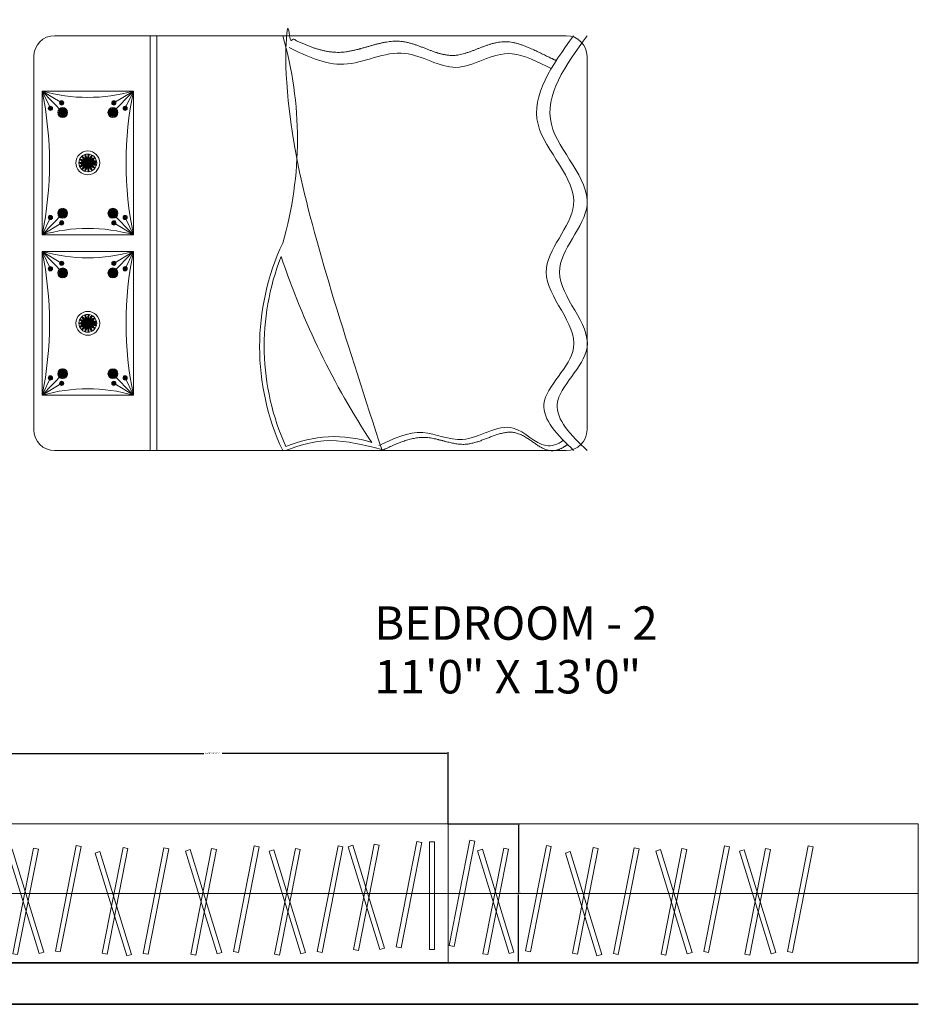
# Model space of a CAD drawing. Units: inches. Extents: x -61 to 1599, y -1316 to 257.
# Tile 74 of 204: x 406 to 536, y -788 to -646. Entities that reach past the tile are written whole.
import ezdxf

# ---------------------------------------------------------------- set-up
doc = ezdxf.new("R2010")
doc.units = ezdxf.units.IN
doc.header["$MEASUREMENT"] = 0
for name, color, linetype, lineweight in [('A-ANNO-DIMS', 2, 'Continuous', 18), ('A-AREA-IDEN', 1, 'Continuous', 18), ('A-FLOR-CASE', 8, 'Continuous', 18), ('FURNITURE', 83, 'Continuous', 18), ('WALLS', 4, 'Continuous', 35)]:
    doc.layers.add(name, color=color, linetype=linetype, lineweight=lineweight)
doc.layers.add('LT', color=8, linetype='Continuous')
doc.styles.get("Standard").update_dxf_attribs({"font": 'arial.ttf'})
doc.dimstyles.get("Standard").update_dxf_attribs({"dimtxt": 0.18, "dimasz": 0.18, "dimexe": 0.18, "dimexo": 0.0625, "dimgap": 0.09, "dimtad": 0, "dimtih": 1, "dimtoh": 1, "dimdec": 0, "dimzin": 0, "dimdsep": 46, "dimlunit": 3, "dimtxsty": 'Standard', "dimcen": 0.09, "dimadec": 0, "dimazin": 0, "dimtfac": 1, "dimtdec": 0, "dimtofl": 0, "dimtmove": 0, "dimatfit": 3, "dimfxl": 1, "dimtolj": 1, "dimtzin": 0, "dimarcsym": 0})

# ---------------------------------------------------------------- blocks, each defined once
blk = doc.blocks.new('*U324')
at = {"layer": 'LT'}
blk.add_line((0, 0.64), (0, -0.64), dxfattribs=at)
for centre, start, end in [((1.87, 0), 160.9983, 199.0017), ((-1.87, 0), 340.9983, 19.0017)]:
    blk.add_arc(centre, 1.97, start, end, dxfattribs=at)
blk = doc.blocks.new('*U311')
at = {"layer": 'FURNITURE', "transparency": 16777216}
for p, rotation in [((-244.2, -68.53), 48.00000000000001), ((-243.98, -68.38), 23.99999999999999), ((-243.46, -68.38), 336.0000000000001), ((-243.25, -68.53), 312), ((-244.36, -69.03), 96), ((-244.33, -68.76), 72), ((-244.28, -69.28), 120), ((-244.1, -69.48), 144), ((-243.86, -69.59), 168), ((-243.59, -69.59), 192), ((-243.34, -69.48), 216), ((-243.17, -69.28), 240), ((-243.11, -68.76), 288), ((-243.08, -69.03), 264)]:
    blk.add_blockref('*U324', p, dxfattribs=dict(at, rotation=rotation))
blk.add_blockref('*U324', (-243.72, -68.32), dxfattribs=at)
blk = doc.blocks.new('*U312')
at = {"layer": 'LT'}
blk.add_line((0, 0.36), (0, -0.36), dxfattribs=at)
for centre, start, end in [((1.04, 0), 160.9983, 199.0017), ((-1.04, 0), 340.9983, 19.0017)]:
    blk.add_arc(centre, 1.1, start, end, dxfattribs=at)
blk = doc.blocks.new('*U313')
at = {"layer": 'FURNITURE', "transparency": 16777216}
for p, rotation in [((-136.32, -38.51), 96), ((-136.3, -38.36), 72), ((-136.27, -38.65), 120), ((-136.23, -38.23), 48.00000000000001), ((-136.17, -38.76), 144), ((-136.11, -38.14), 23.99999999999999), ((-135.82, -38.14), 336.0000000000001), ((-135.75, -38.76), 216), ((-135.69, -38.23), 312), ((-135.65, -38.65), 240), ((-135.62, -38.36), 288.0000000000001), ((-135.6, -38.51), 264), ((-136.04, -38.82), 168.0000000000001), ((-135.89, -38.82), 191.9999999999999)]:
    blk.add_blockref('*U312', p, dxfattribs=dict(at, rotation=rotation))
blk.add_blockref('*U312', (-135.96, -38.11), dxfattribs=at)
blk = doc.blocks.new('*U318')
at = {"layer": 'LT'}
blk.add_line((0, 0.15), (0, -0.15), dxfattribs=at)
for centre, start, end in [((0.44, 0), 160.9983, 199.0017), ((-0.44, 0), 340.9983, 19.0017)]:
    blk.add_arc(centre, 0.468, start, end, dxfattribs=at)
blk = doc.blocks.new('*U319')
at = {"layer": 'FURNITURE', "transparency": 16777216}
for p, rotation in [((-57.96, -16.37), 96), ((-57.96, -16.31), 72), ((-57.94, -16.43), 120), ((-57.93, -16.26), 48.00000000000001), ((-57.9, -16.48), 144), ((-57.87, -16.22), 24), ((-57.84, -16.51), 168.0000000000001), ((-57.75, -16.22), 336), ((-57.78, -16.51), 192), ((-57.7, -16.26), 312), ((-57.72, -16.48), 216), ((-57.68, -16.43), 240), ((-57.67, -16.31), 288), ((-57.66, -16.37), 264)]:
    blk.add_blockref('*U318', p, dxfattribs=dict(at, rotation=rotation))
blk.add_blockref('*U318', (-57.81, -16.21), dxfattribs=at)
blk = doc.blocks.new('*U320')
at = {"layer": 'LT'}
blk.add_line((0, 0.15), (0, -0.15), dxfattribs=at)
for centre, start, end in [((0.44, 0), 160.9983, 199.0017), ((-0.44, 0), 340.9983, 19.0017)]:
    blk.add_arc(centre, 0.468, start, end, dxfattribs=at)
blk = doc.blocks.new('*U321')
at = {"layer": 'FURNITURE', "transparency": 16777216}
for p, rotation in [((-57.96, -16.37), 96), ((-57.96, -16.31), 72), ((-57.94, -16.43), 120), ((-57.93, -16.26), 48.00000000000001), ((-57.9, -16.48), 144), ((-57.87, -16.22), 24), ((-57.84, -16.51), 168.0000000000001), ((-57.75, -16.22), 336), ((-57.78, -16.51), 192), ((-57.7, -16.26), 312), ((-57.72, -16.48), 216), ((-57.68, -16.43), 240), ((-57.67, -16.31), 288), ((-57.66, -16.37), 264)]:
    blk.add_blockref('*U320', p, dxfattribs=dict(at, rotation=rotation))
blk.add_blockref('*U320', (-57.81, -16.21), dxfattribs=at)
blk = doc.blocks.new('*U275')
at = {"layer": 'LT'}
blk.add_line((0, 0.36), (0, -0.36), dxfattribs=at)
for centre, start, end in [((1.04, 0), 160.9983, 199.0017), ((-1.04, 0), 340.9983, 19.0017)]:
    blk.add_arc(centre, 1.1, start, end, dxfattribs=at)
blk = doc.blocks.new('*U317')
at = {"layer": 'FURNITURE', "transparency": 16777216}
for p, rotation in [((-136.32, -38.51), 96), ((-136.3, -38.36), 72), ((-136.27, -38.65), 120), ((-136.23, -38.23), 48.00000000000001), ((-136.17, -38.76), 144), ((-136.11, -38.14), 23.99999999999999), ((-135.82, -38.14), 336.0000000000001), ((-135.75, -38.76), 216), ((-135.69, -38.23), 312), ((-135.65, -38.65), 240), ((-135.62, -38.36), 288.0000000000001), ((-135.6, -38.51), 264), ((-136.04, -38.82), 168.0000000000001), ((-135.89, -38.82), 191.9999999999999)]:
    blk.add_blockref('*U275', p, dxfattribs=dict(at, rotation=rotation))
blk.add_blockref('*U275', (-135.96, -38.11), dxfattribs=at)
blk = doc.blocks.new('*U322')
at = {"layer": 'LT'}
blk.add_line((0, 0.15), (0, -0.15), dxfattribs=at)
for centre, start, end in [((0.44, 0), 160.9983, 199.0017), ((-0.44, 0), 340.9983, 19.0017)]:
    blk.add_arc(centre, 0.468, start, end, dxfattribs=at)
blk = doc.blocks.new('*U323')
at = {"layer": 'FURNITURE', "transparency": 16777216}
for p, rotation in [((-57.96, -16.37), 96), ((-57.96, -16.31), 72), ((-57.94, -16.43), 120), ((-57.93, -16.26), 48.00000000000001), ((-57.9, -16.48), 144), ((-57.87, -16.22), 24), ((-57.84, -16.51), 168.0000000000001), ((-57.75, -16.22), 336), ((-57.78, -16.51), 192), ((-57.7, -16.26), 312), ((-57.72, -16.48), 216), ((-57.68, -16.43), 240), ((-57.67, -16.31), 288), ((-57.66, -16.37), 264)]:
    blk.add_blockref('*U322', p, dxfattribs=dict(at, rotation=rotation))
blk.add_blockref('*U322', (-57.81, -16.21), dxfattribs=at)
blk = doc.blocks.new('*U273')
at = {"layer": 'LT'}
blk.add_line((0, 0.15), (0, -0.15), dxfattribs=at)
for centre, start, end in [((0.44, 0), 160.9983, 199.0017), ((-0.44, 0), 340.9983, 19.0017)]:
    blk.add_arc(centre, 0.468, start, end, dxfattribs=at)
blk = doc.blocks.new('*U274')
at = {"layer": 'FURNITURE', "transparency": 16777216}
for p, rotation in [((-57.96, -16.37), 96), ((-57.96, -16.31), 72), ((-57.94, -16.43), 120), ((-57.93, -16.26), 48.00000000000001), ((-57.9, -16.48), 144), ((-57.87, -16.22), 24), ((-57.84, -16.51), 168.0000000000001), ((-57.75, -16.22), 336), ((-57.78, -16.51), 192), ((-57.7, -16.26), 312), ((-57.72, -16.48), 216), ((-57.68, -16.43), 240), ((-57.67, -16.31), 288), ((-57.66, -16.37), 264)]:
    blk.add_blockref('*U273', p, dxfattribs=dict(at, rotation=rotation))
blk.add_blockref('*U273', (-57.81, -16.21), dxfattribs=at)
blk = doc.blocks.new('*U301')
at = {"layer": 'LT'}
blk.add_line((0, 0.36), (0, -0.36), dxfattribs=at)
for centre, start, end in [((1.04, 0), 160.9983, 199.0017), ((-1.04, 0), 340.9983, 19.0017)]:
    blk.add_arc(centre, 1.1, start, end, dxfattribs=at)
blk = doc.blocks.new('*U302')
at = {"layer": 'FURNITURE', "transparency": 16777216}
for p, rotation in [((-136.32, -38.51), 96), ((-136.3, -38.36), 72), ((-136.27, -38.65), 120), ((-136.23, -38.23), 48.00000000000001), ((-136.17, -38.76), 144), ((-136.11, -38.14), 23.99999999999999), ((-135.82, -38.14), 336.0000000000001), ((-135.75, -38.76), 216), ((-135.69, -38.23), 312), ((-135.65, -38.65), 240), ((-135.62, -38.36), 288.0000000000001), ((-135.6, -38.51), 264), ((-136.04, -38.82), 168.0000000000001), ((-135.89, -38.82), 191.9999999999999)]:
    blk.add_blockref('*U301', p, dxfattribs=dict(at, rotation=rotation))
blk.add_blockref('*U301', (-135.96, -38.11), dxfattribs=at)
blk = doc.blocks.new('*U294')
at = {"layer": 'LT'}
blk.add_line((0, 0.15), (0, -0.15), dxfattribs=at)
for centre, start, end in [((0.44, 0), 160.9983, 199.0017), ((-0.44, 0), 340.9983, 19.0017)]:
    blk.add_arc(centre, 0.468, start, end, dxfattribs=at)
blk = doc.blocks.new('*U295')
at = {"layer": 'FURNITURE', "transparency": 16777216}
for p, rotation in [((-57.96, -16.37), 96), ((-57.96, -16.31), 72), ((-57.94, -16.43), 120), ((-57.93, -16.26), 48.00000000000001), ((-57.9, -16.48), 144), ((-57.87, -16.22), 24), ((-57.84, -16.51), 168.0000000000001), ((-57.75, -16.22), 336), ((-57.78, -16.51), 192), ((-57.7, -16.26), 312), ((-57.72, -16.48), 216), ((-57.68, -16.43), 240), ((-57.67, -16.31), 288), ((-57.66, -16.37), 264)]:
    blk.add_blockref('*U294', p, dxfattribs=dict(at, rotation=rotation))
blk.add_blockref('*U294', (-57.81, -16.21), dxfattribs=at)
blk = doc.blocks.new('*U296')
at = {"layer": 'LT'}
blk.add_line((0, 0.15), (0, -0.15), dxfattribs=at)
for centre, start, end in [((0.44, 0), 160.9983, 199.0017), ((-0.44, 0), 340.9983, 19.0017)]:
    blk.add_arc(centre, 0.468, start, end, dxfattribs=at)
blk = doc.blocks.new('*U297')
at = {"layer": 'FURNITURE', "transparency": 16777216}
for p, rotation in [((-57.96, -16.37), 96), ((-57.96, -16.31), 72), ((-57.94, -16.43), 120), ((-57.93, -16.26), 48.00000000000001), ((-57.9, -16.48), 144), ((-57.87, -16.22), 24), ((-57.84, -16.51), 168.0000000000001), ((-57.75, -16.22), 336), ((-57.78, -16.51), 192), ((-57.7, -16.26), 312), ((-57.72, -16.48), 216), ((-57.68, -16.43), 240), ((-57.67, -16.31), 288), ((-57.66, -16.37), 264)]:
    blk.add_blockref('*U296', p, dxfattribs=dict(at, rotation=rotation))
blk.add_blockref('*U296', (-57.81, -16.21), dxfattribs=at)
blk = doc.blocks.new('*U292')
at = {"layer": 'LT'}
blk.add_line((0, 0.36), (0, -0.36), dxfattribs=at)
for centre, start, end in [((1.04, 0), 160.9983, 199.0017), ((-1.04, 0), 340.9983, 19.0017)]:
    blk.add_arc(centre, 1.1, start, end, dxfattribs=at)
blk = doc.blocks.new('*U293')
at = {"layer": 'FURNITURE', "transparency": 16777216}
for p, rotation in [((-136.32, -38.51), 96), ((-136.3, -38.36), 72), ((-136.27, -38.65), 120), ((-136.23, -38.23), 48.00000000000001), ((-136.17, -38.76), 144), ((-136.11, -38.14), 23.99999999999999), ((-135.82, -38.14), 336.0000000000001), ((-135.75, -38.76), 216), ((-135.69, -38.23), 312), ((-135.65, -38.65), 240), ((-135.62, -38.36), 288.0000000000001), ((-135.6, -38.51), 264), ((-136.04, -38.82), 168.0000000000001), ((-135.89, -38.82), 191.9999999999999)]:
    blk.add_blockref('*U292', p, dxfattribs=dict(at, rotation=rotation))
blk.add_blockref('*U292', (-135.96, -38.11), dxfattribs=at)
blk = doc.blocks.new('*U299')
at = {"layer": 'LT'}
blk.add_line((0, 0.15), (0, -0.15), dxfattribs=at)
for centre, start, end in [((0.44, 0), 160.9983, 199.0017), ((-0.44, 0), 340.9983, 19.0017)]:
    blk.add_arc(centre, 0.468, start, end, dxfattribs=at)
blk = doc.blocks.new('*U300')
at = {"layer": 'FURNITURE', "transparency": 16777216}
for p, rotation in [((-57.96, -16.37), 96), ((-57.96, -16.31), 72), ((-57.94, -16.43), 120), ((-57.93, -16.26), 48.00000000000001), ((-57.9, -16.48), 144), ((-57.87, -16.22), 24), ((-57.84, -16.51), 168.0000000000001), ((-57.75, -16.22), 336), ((-57.78, -16.51), 192), ((-57.7, -16.26), 312), ((-57.72, -16.48), 216), ((-57.68, -16.43), 240), ((-57.67, -16.31), 288), ((-57.66, -16.37), 264)]:
    blk.add_blockref('*U299', p, dxfattribs=dict(at, rotation=rotation))
blk.add_blockref('*U299', (-57.81, -16.21), dxfattribs=at)
blk = doc.blocks.new('*U290')
at = {"layer": 'LT'}
blk.add_line((0, 0.15), (0, -0.15), dxfattribs=at)
for centre, start, end in [((0.44, 0), 160.9983, 199.0017), ((-0.44, 0), 340.9983, 19.0017)]:
    blk.add_arc(centre, 0.468, start, end, dxfattribs=at)
blk = doc.blocks.new('*U291')
at = {"layer": 'FURNITURE', "transparency": 16777216}
for p, rotation in [((-57.96, -16.37), 96), ((-57.96, -16.31), 72), ((-57.94, -16.43), 120), ((-57.93, -16.26), 48.00000000000001), ((-57.9, -16.48), 144), ((-57.87, -16.22), 24), ((-57.84, -16.51), 168.0000000000001), ((-57.75, -16.22), 336), ((-57.78, -16.51), 192), ((-57.7, -16.26), 312), ((-57.72, -16.48), 216), ((-57.68, -16.43), 240), ((-57.67, -16.31), 288), ((-57.66, -16.37), 264)]:
    blk.add_blockref('*U290', p, dxfattribs=dict(at, rotation=rotation))
blk.add_blockref('*U290', (-57.81, -16.21), dxfattribs=at)
blk = doc.blocks.new('*U281')
at = {"layer": 'LT'}
blk.add_line((0, 0.64), (0, -0.64), dxfattribs=at)
for centre, start, end in [((1.87, 0), 160.9983, 199.0017), ((-1.87, 0), 340.9983, 19.0017)]:
    blk.add_arc(centre, 1.97, start, end, dxfattribs=at)
blk = doc.blocks.new('*U282')
at = {"layer": 'FURNITURE', "transparency": 16777216}
for p, rotation in [((-244.2, -68.53), 48.00000000000001), ((-243.98, -68.38), 23.99999999999999), ((-243.46, -68.38), 336.0000000000001), ((-243.25, -68.53), 312), ((-244.36, -69.03), 96), ((-244.33, -68.76), 72), ((-244.28, -69.28), 120), ((-244.1, -69.48), 144), ((-243.86, -69.59), 168), ((-243.59, -69.59), 192), ((-243.34, -69.48), 216), ((-243.17, -69.28), 240), ((-243.11, -68.76), 288), ((-243.08, -69.03), 264)]:
    blk.add_blockref('*U281', p, dxfattribs=dict(at, rotation=rotation))
blk.add_blockref('*U281', (-243.72, -68.32), dxfattribs=at)
blk = doc.blocks.new('*U298')
at = {"layer": 'LT'}
blk.add_line((0, 0.36), (0, -0.36), dxfattribs=at)
for centre, start, end in [((1.04, 0), 160.9983, 199.0017), ((-1.04, 0), 340.9983, 19.0017)]:
    blk.add_arc(centre, 1.1, start, end, dxfattribs=at)
blk = doc.blocks.new('*U314')
at = {"layer": 'FURNITURE', "transparency": 16777216}
for p, rotation in [((-136.32, -38.51), 96), ((-136.3, -38.36), 72), ((-136.27, -38.65), 120), ((-136.23, -38.23), 48.00000000000001), ((-136.17, -38.76), 144), ((-136.11, -38.14), 23.99999999999999), ((-135.82, -38.14), 336.0000000000001), ((-135.75, -38.76), 216), ((-135.69, -38.23), 312), ((-135.65, -38.65), 240), ((-135.62, -38.36), 288.0000000000001), ((-135.6, -38.51), 264), ((-136.04, -38.82), 168.0000000000001), ((-135.89, -38.82), 191.9999999999999)]:
    blk.add_blockref('*U298', p, dxfattribs=dict(at, rotation=rotation))
blk.add_blockref('*U298', (-135.96, -38.11), dxfattribs=at)
blk = doc.blocks.new('*U289')
at = {"layer": 'LT'}
blk.add_line((0, 0.15), (0, -0.15), dxfattribs=at)
for centre, start, end in [((0.44, 0), 160.9983, 199.0017), ((-0.44, 0), 340.9983, 19.0017)]:
    blk.add_arc(centre, 0.468, start, end, dxfattribs=at)
blk = doc.blocks.new('*U276')
at = {"layer": 'FURNITURE', "transparency": 16777216}
for p, rotation in [((-57.96, -16.37), 96), ((-57.96, -16.31), 72), ((-57.94, -16.43), 120), ((-57.93, -16.26), 48.00000000000001), ((-57.9, -16.48), 144), ((-57.87, -16.22), 24), ((-57.84, -16.51), 168.0000000000001), ((-57.75, -16.22), 336), ((-57.78, -16.51), 192), ((-57.7, -16.26), 312), ((-57.72, -16.48), 216), ((-57.68, -16.43), 240), ((-57.67, -16.31), 288), ((-57.66, -16.37), 264)]:
    blk.add_blockref('*U289', p, dxfattribs=dict(at, rotation=rotation))
blk.add_blockref('*U289', (-57.81, -16.21), dxfattribs=at)
blk = doc.blocks.new('*U277')
at = {"layer": 'LT'}
blk.add_line((0, 0.15), (0, -0.15), dxfattribs=at)
for centre, start, end in [((0.44, 0), 160.9983, 199.0017), ((-0.44, 0), 340.9983, 19.0017)]:
    blk.add_arc(centre, 0.468, start, end, dxfattribs=at)
blk = doc.blocks.new('*U278')
at = {"layer": 'FURNITURE', "transparency": 16777216}
for p, rotation in [((-57.96, -16.37), 96), ((-57.96, -16.31), 72), ((-57.94, -16.43), 120), ((-57.93, -16.26), 48.00000000000001), ((-57.9, -16.48), 144), ((-57.87, -16.22), 24), ((-57.84, -16.51), 168.0000000000001), ((-57.75, -16.22), 336), ((-57.78, -16.51), 192), ((-57.7, -16.26), 312), ((-57.72, -16.48), 216), ((-57.68, -16.43), 240), ((-57.67, -16.31), 288), ((-57.66, -16.37), 264)]:
    blk.add_blockref('*U277', p, dxfattribs=dict(at, rotation=rotation))
blk.add_blockref('*U277', (-57.81, -16.21), dxfattribs=at)
blk = doc.blocks.new('*U287')
at = {"layer": 'LT'}
blk.add_line((0, 0.36), (0, -0.36), dxfattribs=at)
for centre, start, end in [((1.04, 0), 160.9983, 199.0017), ((-1.04, 0), 340.9983, 19.0017)]:
    blk.add_arc(centre, 1.1, start, end, dxfattribs=at)
blk = doc.blocks.new('*U288')
at = {"layer": 'FURNITURE', "transparency": 16777216}
for p, rotation in [((-136.32, -38.51), 96), ((-136.3, -38.36), 72), ((-136.27, -38.65), 120), ((-136.23, -38.23), 48.00000000000001), ((-136.17, -38.76), 144), ((-136.11, -38.14), 23.99999999999999), ((-135.82, -38.14), 336.0000000000001), ((-135.75, -38.76), 216), ((-135.69, -38.23), 312), ((-135.65, -38.65), 240), ((-135.62, -38.36), 288.0000000000001), ((-135.6, -38.51), 264), ((-136.04, -38.82), 168.0000000000001), ((-135.89, -38.82), 191.9999999999999)]:
    blk.add_blockref('*U287', p, dxfattribs=dict(at, rotation=rotation))
blk.add_blockref('*U287', (-135.96, -38.11), dxfattribs=at)
blk = doc.blocks.new('*U279')
at = {"layer": 'LT'}
blk.add_line((0, 0.15), (0, -0.15), dxfattribs=at)
for centre, start, end in [((0.44, 0), 160.9983, 199.0017), ((-0.44, 0), 340.9983, 19.0017)]:
    blk.add_arc(centre, 0.468, start, end, dxfattribs=at)
blk = doc.blocks.new('*U280')
at = {"layer": 'FURNITURE', "transparency": 16777216}
for p, rotation in [((-57.96, -16.37), 96), ((-57.96, -16.31), 72), ((-57.94, -16.43), 120), ((-57.93, -16.26), 48.00000000000001), ((-57.9, -16.48), 144), ((-57.87, -16.22), 24), ((-57.84, -16.51), 168.0000000000001), ((-57.75, -16.22), 336), ((-57.78, -16.51), 192), ((-57.7, -16.26), 312), ((-57.72, -16.48), 216), ((-57.68, -16.43), 240), ((-57.67, -16.31), 288), ((-57.66, -16.37), 264)]:
    blk.add_blockref('*U279', p, dxfattribs=dict(at, rotation=rotation))
blk.add_blockref('*U279', (-57.81, -16.21), dxfattribs=at)
blk = doc.blocks.new('*U285')
at = {"layer": 'LT'}
blk.add_line((0, 0.15), (0, -0.15), dxfattribs=at)
for centre, start, end in [((0.44, 0), 160.9983, 199.0017), ((-0.44, 0), 340.9983, 19.0017)]:
    blk.add_arc(centre, 0.468, start, end, dxfattribs=at)
blk = doc.blocks.new('*U286')
at = {"layer": 'FURNITURE', "transparency": 16777216}
for p, rotation in [((-57.96, -16.37), 96), ((-57.96, -16.31), 72), ((-57.94, -16.43), 120), ((-57.93, -16.26), 48.00000000000001), ((-57.9, -16.48), 144), ((-57.87, -16.22), 24), ((-57.84, -16.51), 168.0000000000001), ((-57.75, -16.22), 336), ((-57.78, -16.51), 192), ((-57.7, -16.26), 312), ((-57.72, -16.48), 216), ((-57.68, -16.43), 240), ((-57.67, -16.31), 288), ((-57.66, -16.37), 264)]:
    blk.add_blockref('*U285', p, dxfattribs=dict(at, rotation=rotation))
blk.add_blockref('*U285', (-57.81, -16.21), dxfattribs=at)
blk = doc.blocks.new('*U283')
at = {"layer": 'LT'}
blk.add_line((0, 0.36), (0, -0.36), dxfattribs=at)
for centre, start, end in [((1.04, 0), 160.9983, 199.0017), ((-1.04, 0), 340.9983, 19.0017)]:
    blk.add_arc(centre, 1.1, start, end, dxfattribs=at)
blk = doc.blocks.new('*U284')
at = {"layer": 'FURNITURE', "transparency": 16777216}
for p, rotation in [((-136.32, -38.51), 96), ((-136.3, -38.36), 72), ((-136.27, -38.65), 120), ((-136.23, -38.23), 48.00000000000001), ((-136.17, -38.76), 144), ((-136.11, -38.14), 23.99999999999999), ((-135.82, -38.14), 336.0000000000001), ((-135.75, -38.76), 216), ((-135.69, -38.23), 312), ((-135.65, -38.65), 240), ((-135.62, -38.36), 288.0000000000001), ((-135.6, -38.51), 264), ((-136.04, -38.82), 168.0000000000001), ((-135.89, -38.82), 191.9999999999999)]:
    blk.add_blockref('*U283', p, dxfattribs=dict(at, rotation=rotation))
blk.add_blockref('*U283', (-135.96, -38.11), dxfattribs=at)
blk = doc.blocks.new('*U305')
at = {"layer": 'LT'}
blk.add_line((0, 0.15), (0, -0.15), dxfattribs=at)
for centre, start, end in [((0.44, 0), 160.9983, 199.0017), ((-0.44, 0), 340.9983, 19.0017)]:
    blk.add_arc(centre, 0.468, start, end, dxfattribs=at)
blk = doc.blocks.new('*U306')
at = {"layer": 'FURNITURE', "transparency": 16777216}
for p, rotation in [((-57.96, -16.37), 96), ((-57.96, -16.31), 72), ((-57.94, -16.43), 120), ((-57.93, -16.26), 48.00000000000001), ((-57.9, -16.48), 144), ((-57.87, -16.22), 24), ((-57.84, -16.51), 168.0000000000001), ((-57.75, -16.22), 336), ((-57.78, -16.51), 192), ((-57.7, -16.26), 312), ((-57.72, -16.48), 216), ((-57.68, -16.43), 240), ((-57.67, -16.31), 288), ((-57.66, -16.37), 264)]:
    blk.add_blockref('*U305', p, dxfattribs=dict(at, rotation=rotation))
blk.add_blockref('*U305', (-57.81, -16.21), dxfattribs=at)
blk = doc.blocks.new('*U307')
at = {"layer": 'LT'}
blk.add_line((0, 0.15), (0, -0.15), dxfattribs=at)
for centre, start, end in [((0.44, 0), 160.9983, 199.0017), ((-0.44, 0), 340.9983, 19.0017)]:
    blk.add_arc(centre, 0.468, start, end, dxfattribs=at)
blk = doc.blocks.new('*U308')
at = {"layer": 'FURNITURE', "transparency": 16777216}
for p, rotation in [((-57.96, -16.37), 96), ((-57.96, -16.31), 72), ((-57.94, -16.43), 120), ((-57.93, -16.26), 48.00000000000001), ((-57.9, -16.48), 144), ((-57.87, -16.22), 24), ((-57.84, -16.51), 168.0000000000001), ((-57.75, -16.22), 336), ((-57.78, -16.51), 192), ((-57.7, -16.26), 312), ((-57.72, -16.48), 216), ((-57.68, -16.43), 240), ((-57.67, -16.31), 288), ((-57.66, -16.37), 264)]:
    blk.add_blockref('*U307', p, dxfattribs=dict(at, rotation=rotation))
blk.add_blockref('*U307', (-57.81, -16.21), dxfattribs=at)
blk = doc.blocks.new('*U303')
at = {"layer": 'LT'}
blk.add_line((0, 0.36), (0, -0.36), dxfattribs=at)
for centre, start, end in [((1.04, 0), 160.9983, 199.0017), ((-1.04, 0), 340.9983, 19.0017)]:
    blk.add_arc(centre, 1.1, start, end, dxfattribs=at)
blk = doc.blocks.new('*U304')
at = {"layer": 'FURNITURE', "transparency": 16777216}
for p, rotation in [((-136.32, -38.51), 96), ((-136.3, -38.36), 72), ((-136.27, -38.65), 120), ((-136.23, -38.23), 48.00000000000001), ((-136.17, -38.76), 144), ((-136.11, -38.14), 23.99999999999999), ((-135.82, -38.14), 336.0000000000001), ((-135.75, -38.76), 216), ((-135.69, -38.23), 312), ((-135.65, -38.65), 240), ((-135.62, -38.36), 288.0000000000001), ((-135.6, -38.51), 264), ((-136.04, -38.82), 168.0000000000001), ((-135.89, -38.82), 191.9999999999999)]:
    blk.add_blockref('*U303', p, dxfattribs=dict(at, rotation=rotation))
blk.add_blockref('*U303', (-135.96, -38.11), dxfattribs=at)
blk = doc.blocks.new('*U309')
at = {"layer": 'LT'}
blk.add_line((0, 0.15), (0, -0.15), dxfattribs=at)
for centre, start, end in [((0.44, 0), 160.9983, 199.0017), ((-0.44, 0), 340.9983, 19.0017)]:
    blk.add_arc(centre, 0.468, start, end, dxfattribs=at)
blk = doc.blocks.new('*U310')
at = {"layer": 'FURNITURE', "transparency": 16777216}
for p, rotation in [((-57.96, -16.37), 96), ((-57.96, -16.31), 72), ((-57.94, -16.43), 120), ((-57.93, -16.26), 48.00000000000001), ((-57.9, -16.48), 144), ((-57.87, -16.22), 24), ((-57.84, -16.51), 168.0000000000001), ((-57.75, -16.22), 336), ((-57.78, -16.51), 192), ((-57.7, -16.26), 312), ((-57.72, -16.48), 216), ((-57.68, -16.43), 240), ((-57.67, -16.31), 288), ((-57.66, -16.37), 264)]:
    blk.add_blockref('*U309', p, dxfattribs=dict(at, rotation=rotation))
blk.add_blockref('*U309', (-57.81, -16.21), dxfattribs=at)
blk = doc.blocks.new('*U315')
at = {"layer": 'LT'}
blk.add_line((0, 0.15), (0, -0.15), dxfattribs=at)
for centre, start, end in [((0.44, 0), 160.9983, 199.0017), ((-0.44, 0), 340.9983, 19.0017)]:
    blk.add_arc(centre, 0.468, start, end, dxfattribs=at)
blk = doc.blocks.new('*U316')
at = {"layer": 'FURNITURE', "transparency": 16777216}
for p, rotation in [((-57.96, -16.37), 96), ((-57.96, -16.31), 72), ((-57.94, -16.43), 120), ((-57.93, -16.26), 48.00000000000001), ((-57.9, -16.48), 144), ((-57.87, -16.22), 24), ((-57.84, -16.51), 168.0000000000001), ((-57.75, -16.22), 336), ((-57.78, -16.51), 192), ((-57.7, -16.26), 312), ((-57.72, -16.48), 216), ((-57.68, -16.43), 240), ((-57.67, -16.31), 288), ((-57.66, -16.37), 264)]:
    blk.add_blockref('*U315', p, dxfattribs=dict(at, rotation=rotation))
blk.add_blockref('*U315', (-57.81, -16.21), dxfattribs=at)
blk = doc.blocks.new('WARDROBE-HANGING')
blk.add_line((10.05, 0), (10.05, 68))
for points in [[(20.09, 0), (0, 0), (0, 68), (20.09, 68)], [(2.48, 67.85), (17.75, 64.85), (17.61, 64.14), (2.34, 67.15)], [(1.32, 62.96), (16.59, 59.95), (16.45, 59.25), (1.19, 62.25)], [(1.35, 59.16), (16.22, 63.73), (16.43, 63.04), (1.56, 58.47)], [(1.71, 56.78), (16.98, 53.78), (16.84, 53.07), (1.57, 56.08)], [(1, 46.47), (15.87, 51.04), (16.08, 50.35), (1.21, 45.78)], [(1.39, 50.01), (16.66, 47.01), (16.52, 46.3), (1.26, 49.31)], [(1.36, 44.09), (16.63, 41.09), (16.49, 40.38), (1.23, 43.38)], [(1.26, 37.2), (16.53, 34.2), (16.39, 33.49), (1.12, 36.5)], [(1.28, 33.41), (16.16, 37.98), (16.37, 37.29), (1.49, 32.72)], [(1.65, 31.03), (16.92, 28.03), (16.78, 27.32), (1.51, 30.32)], [(1.28, 21.3), (16.15, 25.87), (16.36, 25.18), (1.49, 20.61)], [(1.26, 25.09), (16.53, 22.09), (16.39, 21.38), (1.12, 24.39)], [(1.65, 18.92), (16.91, 15.92), (16.78, 15.21), (1.51, 18.21)], [(1.93, 9.89), (16.8, 14.46), (17.01, 13.77), (2.14, 9.2)], [(1.91, 13.69), (17.17, 10.68), (17.04, 9.98), (1.77, 12.98)], [(2.29, 7.51), (17.56, 4.51), (17.42, 3.8), (2.16, 6.81)], [(17.49, 1.96), (1.93, 1.96), (1.93, 2.68), (17.49, 2.68)]]:
    blk.add_lwpolyline(points, close=True)
blk = doc.blocks.new('*D620')
at = {"layer": 'A-ANNO-DIMS', "color": 0, "lineweight": -2, "transparency": 16777216}
for p, q in [((399.7, -761.79), (399.7, -751.47)), ((399.88, -751.65), (432.4, -751.65)), ((467.52, -751.65), (435.01, -751.65)), ((467.7, -761.79), (467.7, -751.47))]:
    blk.add_line(p, q, dxfattribs=at)
at = {"layer": 'A-ANNO-DIMS', "color": 0, "transparency": 16777216}
for points in [[(399.88, -751.62), (399.88, -751.68), (399.7, -751.65)], [(467.52, -751.62), (467.52, -751.68), (467.7, -751.65)]]:
    blk.add_solid(points, dxfattribs=at)
at = {"layer": 'DEFPOINTS', "color": 0, "transparency": 16777216}
for p in [(399.7, -751.65), (399.7, -761.85), (467.7, -761.85)]:
    blk.add_point(p, dxfattribs=at)
at = {"layer": 'A-ANNO-DIMS', "color": 0, "transparency": 16777216, "insert": (433.7, -751.65), "char_height": 0.18, "attachment_point": 5}
blk.add_mtext('\\A1;WARDROBE 68 TYP.', dxfattribs=at)
blk = doc.blocks.new('*D621')
at = {"layer": 'A-ANNO-DIMS', "color": 0, "lineweight": -2, "transparency": 16777216}
for p, q in [((467.77, -761.85), (478.08, -761.85)), ((477.9, -762.03), (477.9, -771.72)), ((477.9, -781.76), (477.9, -772.08)), ((467.77, -781.94), (478.08, -781.94))]:
    blk.add_line(p, q, dxfattribs=at)
at = {"layer": 'A-ANNO-DIMS', "color": 0, "transparency": 16777216}
for points in [[(477.87, -762.03), (477.93, -762.03), (477.9, -761.85)], [(477.87, -781.76), (477.93, -781.76), (477.9, -781.94)]]:
    blk.add_solid(points, dxfattribs=at)
at = {"layer": 'DEFPOINTS', "color": 0, "transparency": 16777216}
for p in [(467.7, -761.85), (477.9, -761.85), (467.7, -781.94)]:
    blk.add_point(p, dxfattribs=at)
at = {"layer": 'A-ANNO-DIMS', "color": 0, "transparency": 16777216, "insert": (477.9, -771.9), "char_height": 0.18, "attachment_point": 5}
blk.add_mtext('\\A1;20 TYP.', dxfattribs=at)

msp = doc.modelspace()

# ---------------------------------------------------------------- linework, layer by layer
at = {"layer": 'A-FLOR-CASE'}
msp.add_line((535.7028, -771.8978), (467.7028, -771.8978), dxfattribs=at)
for points in [[(535.7028, -761.851), (535.7028, -781.9446), (467.7028, -781.9446), (467.7028, -761.851)], [(467.8507, -779.4624), (470.8541, -764.1942), (471.5606, -764.3332), (468.5572, -779.6014)], [(476.5411, -780.5988), (471.972, -765.7239), (472.6602, -765.5125), (477.2293, -780.3874)], [(472.7457, -780.6203), (475.7491, -765.3521), (476.4555, -765.4911), (473.4521, -780.7592)], [(478.9186, -780.2316), (481.922, -764.9634), (482.6285, -765.1023), (479.625, -780.3705)], [(489.2357, -780.9475), (484.6665, -766.0726), (485.3547, -765.8612), (489.9239, -780.7361)], [(485.6884, -780.5508), (488.6918, -765.2826), (489.3982, -765.4216), (486.3948, -780.6898)], [(491.6132, -780.5802), (494.6166, -765.312), (495.323, -765.451), (492.3196, -780.7192)], [(502.2951, -780.6614), (497.726, -765.7866), (498.4142, -765.5752), (502.9834, -780.45)], [(498.4998, -780.6829), (501.5032, -765.4147), (502.2096, -765.5537), (499.2062, -780.8219)], [(504.6727, -780.2942), (507.6761, -765.026), (508.3825, -765.165), (505.3791, -780.4331)], [(514.4041, -780.6661), (509.8349, -765.7912), (510.5232, -765.5798), (515.0923, -780.4547)], [(510.6087, -780.6876), (513.6121, -765.4194), (514.3185, -765.5583), (511.3151, -780.8265)], [(516.7816, -780.2988), (519.785, -765.0307), (520.4914, -765.1696), (517.488, -780.4378)]]:
    msp.add_lwpolyline(points, close=True, dxfattribs=at)
at = {"layer": 'FURNITURE'}
for p, q in [((424.5945, -647.8524), (424.5945, -707.8524)), ((425.5945, -647.8524), (425.5945, -707.8524)), ((408.9945, -655.8524), (422.1945, -655.8524)), ((408.9945, -655.8524), (410.1921, -658.3566)), ((408.9945, -655.8524), (411.9954, -658.9552)), ((408.9945, -655.8524), (411.8225, -657.5768)), ((422.1945, -655.8524), (419.1935, -658.9552)), ((422.1945, -655.8524), (419.3664, -657.5768)), ((422.1945, -655.8524), (420.9968, -658.3566)), ((422.1945, -676.6524), (422.1945, -655.8524)), ((411.8225, -657.5768), (412.1275, -657.5768)), ((419.3664, -657.5768), (419.0614, -657.5768)), ((410.1921, -658.3566), (410.4971, -658.3566)), ((411.9588, -658.9671), (412.676, -658.9671)), ((419.2302, -658.9671), (418.5129, -658.9671)), ((420.9968, -658.3566), (420.6918, -658.3566)), ((415.5945, -666.2524), (416.8802, -666.2524)), ((408.9945, -676.6524), (411.9954, -673.5496)), ((411.9588, -673.5377), (412.676, -673.5377)), ((419.2302, -673.5377), (418.5129, -673.5377)), ((422.1945, -676.6524), (419.1935, -673.5496)), ((408.9945, -676.6524), (410.1921, -674.1482)), ((408.9945, -676.6524), (411.8225, -674.928)), ((410.1921, -674.1482), (410.4971, -674.1482)), ((411.8225, -674.928), (412.1275, -674.928)), ((419.3664, -674.928), (419.0614, -674.928)), ((422.1945, -676.6524), (419.3664, -674.928)), ((420.9968, -674.1482), (420.6918, -674.1482)), ((422.1945, -676.6524), (420.9968, -674.1482)), ((408.9945, -676.6524), (408.9945, -676.6524)), ((408.9945, -679.0524), (422.1945, -679.0524)), ((408.9945, -679.0524), (410.1921, -681.5566)), ((408.9945, -679.0524), (411.9954, -682.1552)), ((408.9945, -679.0524), (411.8225, -680.7768)), ((422.1945, -679.0524), (419.1935, -682.1552)), ((422.1945, -679.0524), (419.3664, -680.7768)), ((422.1945, -679.0524), (420.9968, -681.5566)), ((422.1945, -699.8524), (422.1945, -679.0524)), ((410.1921, -681.5566), (410.4971, -681.5566)), ((411.8225, -680.7768), (412.1275, -680.7768)), ((419.3664, -680.7768), (419.0614, -680.7768)), ((420.9968, -681.5566), (420.6918, -681.5566)), ((411.9588, -682.1671), (412.676, -682.1671)), ((419.2302, -682.1671), (418.5129, -682.1671)), ((415.5945, -689.4524), (416.8802, -689.4524)), ((408.9945, -699.8524), (411.9954, -696.7496)), ((408.9945, -699.8524), (410.1921, -697.3482)), ((410.1921, -697.3482), (410.4971, -697.3482)), ((411.9588, -696.7377), (412.676, -696.7377)), ((419.2302, -696.7377), (418.5129, -696.7377)), ((422.1945, -699.8524), (419.1935, -696.7496)), ((420.9968, -697.3482), (420.6918, -697.3482)), ((422.1945, -699.8524), (420.9968, -697.3482)), ((408.9945, -699.8524), (411.8225, -698.128)), ((411.8225, -698.128), (412.1275, -698.128)), ((419.3664, -698.128), (419.0614, -698.128)), ((422.1945, -699.8524), (419.3664, -698.128)), ((408.9945, -699.8524), (408.9945, -699.8524))]:
    msp.add_line(p, q, dxfattribs=at)
for points in [[(484.7945, -647.8524), (410.7945, -647.8524, 0.41421356), (407.7945, -650.8524), (407.7945, -704.8524, 0.41421356), (410.7945, -707.8524), (484.7945, -707.8524, 0.41421356), (487.7945, -704.8524), (487.7945, -650.8524, 0.41421356)], [(412.1275, -657.5768, 0.16735782), (411.8225, -657.5768, 0.16735782)], [(419.3664, -657.5768, 0.16735782), (419.0614, -657.5768, 0.16735782)], [(410.4971, -658.3566, 0.16735782), (410.1921, -658.3566, 0.16735782)], [(412.676, -658.9671, 0.16735782), (411.9588, -658.9671, 0.16735782)], [(419.2302, -658.9671, 0.16735782), (418.5129, -658.9671, 0.16735782)], [(420.9968, -658.3566, 0.16735782), (420.6918, -658.3566, 0.16735782)], [(415.5945, -666.2524, 0.16735782), (416.8802, -666.2524, 0.16735782)], [(411.9588, -673.5377, 0.16735782), (412.676, -673.5377, 0.16735782)], [(418.5129, -673.5377, 0.16735782), (419.2302, -673.5377, 0.16735782)], [(410.1921, -674.1482, 0.16735782), (410.4971, -674.1482, 0.16735782)], [(411.8225, -674.928, 0.16735782), (412.1275, -674.928, 0.16735782)], [(419.0614, -674.928, 0.16735782), (419.3664, -674.928, 0.16735782)], [(443.5615, -679.8029, 0.0643962), (456.6549, -706.696, 0.18176597), (444.249, -707.288, -0.20276739)], [(410.4971, -681.5566, 0.16735782), (410.1921, -681.5566, 0.16735782)], [(412.1275, -680.7768, 0.16735782), (411.8225, -680.7768, 0.16735782)], [(412.676, -682.1671, 0.16735782), (411.9588, -682.1671, 0.16735782)], [(419.2302, -682.1671, 0.16735782), (418.5129, -682.1671, 0.16735782)], [(419.3664, -680.7768, 0.16735782), (419.0614, -680.7768, 0.16735782)], [(420.9968, -681.5566, 0.16735782), (420.6918, -681.5566, 0.16735782)], [(415.5945, -689.4524, 0.16735782), (416.8802, -689.4524, 0.16735782)], [(410.1921, -697.3482, 0.16735782), (410.4971, -697.3482, 0.16735782)], [(411.9588, -696.7377, 0.16735782), (412.676, -696.7377, 0.16735782)], [(418.5129, -696.7377, 0.16735782), (419.2302, -696.7377, 0.16735782)], [(411.8225, -698.128, 0.16735782), (412.1275, -698.128, 0.16735782)], [(419.0614, -698.128, 0.16735782), (419.3664, -698.128, 0.16735782)]]:
    msp.add_lwpolyline(points, format="xyb", close=True, dxfattribs=at)
msp.add_lwpolyline([(443.789, -707.8524, -0.22309038), (443.789, -677.8524, 0.14215569), (443.789, -647.8524)], format="xyb", dxfattribs=at)
for points in [[(422.1945, -676.6524), (408.9945, -676.6524), (408.9945, -655.8524), (422.1945, -655.8524), (422.1945, -676.6524), (408.9945, -676.6524), (408.9945, -655.8524)], [(422.1945, -699.8524), (408.9945, -699.8524), (408.9945, -679.0524)]]:
    msp.add_lwpolyline(points, dxfattribs=at)
for centre, radius in [((411.8225, -657.5768), 0.305), ((419.3664, -657.5768), 0.305), ((410.1921, -658.3566), 0.305), ((411.9588, -658.9671), 0.7173), ((419.2302, -658.9671), 0.7173), ((420.9968, -658.3566), 0.305), ((415.5945, -666.2524), 1.7241), ((415.5945, -666.2524), 1.2858), ((411.9588, -673.5377), 0.7173), ((419.2302, -673.5377), 0.7173), ((410.1921, -674.1482), 0.305), ((411.8225, -674.928), 0.305), ((419.3664, -674.928), 0.305), ((420.9968, -674.1482), 0.305), ((411.8225, -680.7768), 0.305), ((419.3664, -680.7768), 0.305), ((410.1921, -681.5566), 0.305), ((411.9588, -682.1671), 0.7173), ((419.2302, -682.1671), 0.7173), ((420.9968, -681.5566), 0.305), ((415.5945, -689.4524), 1.7241), ((415.5945, -689.4524), 1.2858), ((411.9588, -696.7377), 0.7173), ((419.2302, -696.7377), 0.7173), ((410.1921, -697.3482), 0.305), ((420.9968, -697.3482), 0.305), ((411.8225, -698.128), 0.305), ((419.3664, -698.128), 0.305)]:
    msp.add_circle(centre, radius, dxfattribs=at)
for centre, radius, start, end in [((358.5675, -666.2524), 51.4883, 348.34678, 11.65322), ((415.5945, -632.8285), 23.9512, 254.004596, 285.995404), ((472.6214, -666.2524), 51.4883, 168.34678, 191.65322), ((420.8443, -674.5911), 0.4684, 70.998304, 109.001696), ((420.8443, -673.7054), 0.4684, 250.998304, 289.001696), ((415.5945, -699.6763), 23.9512, 74.004596, 105.995404), ((358.5675, -689.4524), 51.4883, 348.34678, 11.65322), ((415.5945, -656.0285), 23.9512, 254.004596, 285.995404), ((472.6214, -689.4524), 51.4883, 168.34678, 191.65322), ((420.8443, -697.7911), 0.4684, 70.998304, 109.001696), ((420.8443, -696.9054), 0.4684, 250.998304, 289.001696), ((415.5945, -722.8763), 23.9512, 74.004596, 105.995404)]:
    msp.add_arc(centre, radius, start, end, dxfattribs=at)
for points, weights, knots in [([(458.15, -707.8524), (452.0994, -698.8072), (447.3656, -689.0084), (444.0407, -678.6465), (444.1229, -678.4576), (444.2068, -678.2694), (444.2923, -678.082), (447.1778, -668.1379), (447.1548, -657.7836), (444.2251, -647.8524), (446.8436, -649.1139), (452.2984, -651.7418), (460.5867, -646.8651), (468.6482, -652.6844), (475.4453, -646.8405), (481.1816, -650.5324), (483.3499, -651.4401)], [1, 0.993520320424, 0.993520320424, 1, 0.99997444972, 0.99997444972, 1, 0.973174868659, 0.973174868659, 1, 1, 1, 1, 1, 1, 1, 1], [0, 0, 0, 0, 0.27907426, 0.27907426, 0.27907426, 0.29658441, 0.29658441, 0.29658441, 0.865868, 0.865868, 0.865868, 9.14257782, 18.10773356, 25.76922649, 34.11080071, 40.44151071, 40.44151071, 40.44151071, 40.44151071]), ([(444.1696, -707.8524), (448.6954, -705.8999), (453.6243, -705.8999), (458.15, -707.8524), (460.2614, -706.8416), (464.215, -704.949), (470.7983, -708.3671), (477.0655, -703.2137), (481.7104, -708.6556), (484.0901, -707.6361), (484.9714, -706.9739)], [1, 0.945466318698, 0.945466318698, 1, 1, 1, 1, 1, 1, 1, 1], [0, 0, 0, 0, 0.81457095, 0.81457095, 0.81457095, 7.46424718, 13.26635305, 20.78853735, 26.13874538, 29.32189524, 29.32189524, 29.32189524, 29.32189524])]:
    msp.add_rational_spline(points, weights, degree=3, knots=knots, dxfattribs=at)
for points, knots in [([(485.8621, -707.8524), (483.5939, -705.63), (478.711, -700.8456), (489.9823, -692.3934), (477.8216, -682.3331), (489.9936, -671.6265), (476.7655, -660.3952), (482.7508, -652.1423), (485.8621, -647.8524)], [0, 0, 0, 0, 7.98028474, 17.17980625, 28.83027828, 39.31808444, 52.07826355, 65.89154622, 65.89154622, 65.89154622, 65.89154622]), ([(487.7945, -707.8524), (485.5263, -705.63), (480.6434, -700.8456), (491.9147, -692.3934), (479.754, -682.3331), (491.926, -671.6265), (478.6979, -660.3952), (484.6832, -652.1423), (487.7945, -647.8524)], [0, 0, 0, 0, 7.98028474, 17.17980625, 28.83027828, 39.31808444, 52.07826355, 65.89154622, 65.89154622, 65.89154622, 65.89154622]), ([(444.702, -649.5738), (447.3205, -650.8353), (452.7753, -653.4632), (461.0636, -648.5865), (469.1251, -654.4058), (475.5727, -648.8624), (480.7683, -651.722), (482.6198, -652.6124)], [0, 0, 0, 0, 8.27670983, 17.24186556, 24.90335849, 33.24493271, 38.42729402, 38.42729402, 38.42729402, 38.42729402]), ([(457.6818, -707.1469), (459.7932, -706.1362), (463.7468, -704.2435), (470.3301, -707.6616), (476.5973, -702.5082), (481.1966, -707.8968), (483.534, -706.9669), (484.3722, -706.3647)], [0, 0, 0, 0, 6.64967623, 12.4517821, 19.9739664, 25.32417443, 28.34967573, 28.34967573, 28.34967573, 28.34967573])]:
    msp.add_open_spline(points, degree=3, knots=knots, dxfattribs=at)
msp.add_open_spline([(487.7945, -651.1038), (487.8113, -651.0823), (487.8279, -651.0603), (487.8445, -651.0384)], degree=3, dxfattribs=at)
at = {"layer": 'WALLS'}
for p, q in [((397.7028, -781.9446), (535.7028, -781.9446)), ((397.7028, -787.9446), (535.7028, -787.9446))]:
    msp.add_line(p, q, dxfattribs=at)

# ---------------------------------------------------------------- block references
at = {"layer": 'A-FLOR-CASE', "rotation": 90.00000000000078}
msp.add_blockref('WARDROBE-HANGING', (467.7029, -781.9448), dxfattribs=at)
at = {"layer": 'FURNITURE', "xscale": -1}
for name, p, rotation in [('*U286', (395.4641, -715.3894), 90), ('*U280', (393.8338, -716.1691), 90), ('*U288', (373.4879, -794.928), 90), ('*U284', (457.701, -537.5768), 270), ('*U308', (435.7248, -617.1154), 270), ('*U306', (437.3552, -616.3357), 270), ('*U274', (395.4641, -738.5894), 90), ('*U323', (393.8338, -739.3691), 90), ('*U317', (373.4879, -818.128), 90), ('*U302', (457.701, -560.7768), 270), ('*U295', (437.3552, -639.5357), 270), ('*U297', (435.7248, -640.3154), 270)]:
    msp.add_blockref(name, p, dxfattribs=dict(at, rotation=rotation))
at = {"layer": 'FURNITURE'}
for name, p, rotation in [('*U316', (435.7248, -715.3894), 270), ('*U304', (457.701, -794.928), 270), ('*U310', (437.3552, -716.1691), 270), ('*U282', (346.6319, -422.5296), 89.99999999999999), ('*U314', (373.4879, -537.5768), 89.99999999999999), ('*U276', (393.8338, -616.3357), 89.99999999999999), ('*U278', (395.4641, -617.1154), 89.99999999999999), ('*U291', (435.7248, -738.5894), 270), ('*U293', (457.701, -818.128), 270), ('*U300', (437.3552, -739.3691), 270), ('*U311', (346.6319, -445.7296), 89.99999999999999), ('*U313', (373.4879, -560.7768), 89.99999999999999), ('*U319', (393.8338, -639.5357), 89.99999999999999), ('*U321', (395.4641, -640.3154), 89.99999999999999)]:
    msp.add_blockref(name, p, dxfattribs=dict(at, rotation=rotation))

# ---------------------------------------------------------------- texts
at = {"layer": 'A-AREA-IDEN'}
for s, p in [('BEDROOM - 2', (457.0332, -735.2211)), ('11\'0" X 13\'0"', (457.0332, -742.9834))]:
    msp.add_text(s, height=4.832098, dxfattribs=at).set_placement(p)

# ---------------------------------------------------------------- dimensions: what is measured, and where the dimension line sits
at = {"layer": 'A-ANNO-DIMS'}
for base, p1, p2, angle, text, picture, middle in [((399.7028, -751.651), (467.7028, -761.851), (399.7028, -761.851), 180, 'WARDROBE <> TYP.', '*D620', (433.7028, -751.651)), ((477.9028, -761.851), (467.7028, -781.9446), (467.7028, -761.851), 90, '<> TYP.', '*D621', (477.9028, -771.8978))]:
    dim = msp.add_linear_dim(base=base, p1=p1, p2=p2, angle=angle, text=text, dimstyle='Standard', override={"dimdec": 0, "dimlfac": 1, "dimrnd": 0, "dimzin": 0, "dimdsep": 46, "dimlunit": 2}, dxfattribs=at)
    dim.commit()
    dim.dimension.update_dxf_attribs({"geometry": picture, "text_midpoint": middle})

doc.saveas('drawing.dxf')
